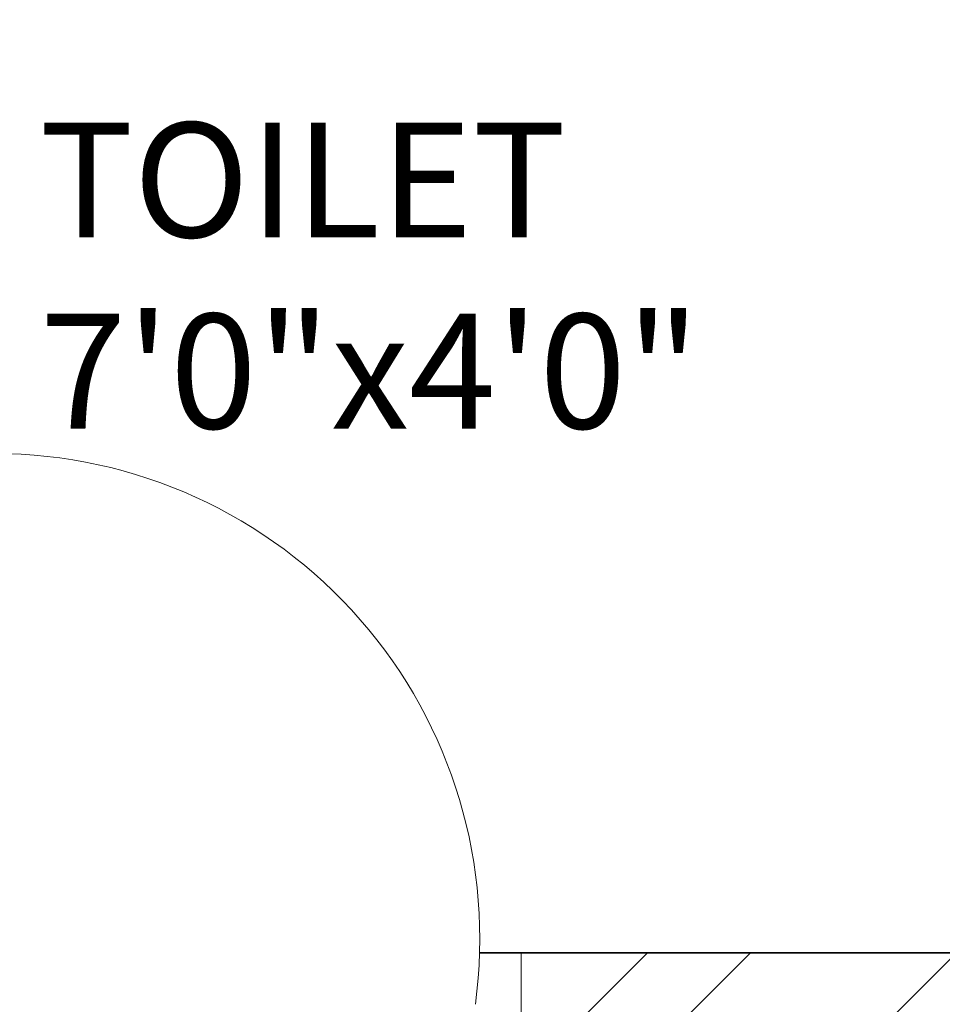
# Model space of a CAD drawing. Units: inches. Extents: x 1962 to 2771, y 1245 to 2660.
# Tile 16 of 114: x 2580 to 2621, y 1649 to 1692. Entities that reach past the tile are written whole.
import ezdxf

# ---------------------------------------------------------------- set-up
doc = ezdxf.new("R2010")
doc.units = ezdxf.units.IN
for name, color, linetype, lineweight in [('A-AREA-IDEN', 7, 'Continuous', 18), ('A-DOOR', 3, 'Continuous', 18), ('A-WALL', 7, 'Continuous', 35), ('A-WALL-PATT', 252, 'Continuous', 13)]:
    doc.layers.add(name, color=color, linetype=linetype, lineweight=lineweight)
doc.styles.get("Standard").update_dxf_attribs({"font": 'arial.ttf'})

msp = doc.modelspace()

# ---------------------------------------------------------------- hatches: boundary and pattern name
at = {"layer": 'A-WALL-PATT'}
h = msp.add_hatch(dxfattribs=at)
h.set_pattern_fill('ANSI32', color=256)
h.paths.add_polyline_path([(2090.8074, 2467.3437), (2141.6481, 2467.3437), (2141.6481, 2469.5937), (2141.6481, 2471.8437), (2086.3074, 2471.8437), (2086.3074, 2422.5333), (2090.8074, 2422.5333)])
h.paths.add_polyline_path([(2282.7664, 2471.8437), (2204.8982, 2471.8437), (2204.8982, 2467.3437), (2234.8074, 2467.3437), (2234.8074, 2311.3437), (2228.7492, 2311.3437), (2228.7492, 2306.8437), (2234.8074, 2306.8437), (2331.9227, 2306.8437), (2331.9227, 2309.0937), (2331.9227, 2311.3437), (2239.3074, 2311.3437), (2239.3074, 2467.3437), (2282.7664, 2467.3437), (2282.7664, 2469.5937)])
h.paths.add_polyline_path([(2471.4531, 2519.8437), (2552.011, 2519.8437), (2564.3996, 2519.8437), (2564.3996, 2511.1389), (2568.8996, 2511.1389), (2568.8996, 2524.3437), (2466.9531, 2524.3437), (2466.9531, 2471.8437), (2450.0749, 2471.8437), (2446.4672, 2471.8437), (2446.4672, 2467.3437), (2450.0749, 2467.3437), (2475.9988, 2467.3437), (2475.9988, 2469.5937), (2475.9988, 2471.8437), (2471.4531, 2471.8437)])
h.paths.add_polyline_path([(2575.2231, 2469.5937), (2575.2231, 2471.8437), (2568.8996, 2471.8437), (2568.8996, 2487.1389), (2564.3996, 2487.1389), (2564.3996, 2471.8437), (2556.511, 2471.8437), (2499.2904, 2471.8437), (2499.2904, 2467.3437), (2507.8074, 2467.3437), (2507.8074, 2311.3437), (2414.863, 2311.3437), (2414.863, 2306.8437), (2512.3074, 2306.8437), (2517.0114, 2306.8437), (2517.0114, 2309.0937), (2517.0114, 2311.3437), (2512.3074, 2311.3437), (2512.3074, 2467.3437), (2575.2231, 2467.3437)])
h.paths.add_polyline_path([(2660.8074, 2471.8437), (2600.9602, 2471.8437), (2600.9602, 2467.3437), (2656.3074, 2467.3437), (2656.3074, 2432.5704), (2660.8074, 2432.5704)])
h.paths.add_polyline_path([(2660.8074, 2372.5704), (2656.3074, 2372.5704), (2656.3074, 2311.3437), (2600.276, 2311.3437), (2600.276, 2309.0937), (2600.276, 2306.8437), (2656.3074, 2306.8437), (2656.3074, 2296.2593), (2660.8074, 2296.2593)])
h.paths.add_polyline_path([(2572.3074, 2306.8437), (2577.1385, 2306.8437), (2577.1385, 2311.3437), (2551.082, 2311.3437), (2551.082, 2306.8437), (2567.8074, 2306.8437), (2567.8074, 2258.8437), (2540.0574, 2258.8437), (2540.0574, 2256.5937), (2540.0574, 2254.3437), (2567.8074, 2254.3437), (2656.3074, 2254.3437), (2656.3074, 2236.9085), (2660.8074, 2236.9085), (2660.8074, 2272.2593), (2656.3074, 2272.2593), (2656.3074, 2258.8437), (2572.3074, 2258.8437)])
h.paths.add_polyline_path([(2512.3074, 2254.3437), (2518.8716, 2254.3437), (2518.8716, 2256.5937), (2518.8716, 2258.8437), (2507.8074, 2258.8437), (2507.8074, 2177.8437), (2567.8074, 2177.8437), (2567.8074, 2172.9628), (2572.3074, 2172.9628), (2572.3074, 2177.8437), (2656.3074, 2177.8437), (2656.3074, 2166.4846), (2660.8074, 2166.4846), (2660.8074, 2200.9085), (2656.3074, 2200.9085), (2656.3074, 2182.3437), (2512.3074, 2182.3437)])
h.paths.add_polyline_path([(2656.3074, 2129.8437), (2572.3074, 2129.8437), (2572.3074, 2150.3044), (2570.0574, 2150.3044), (2567.8074, 2150.3044), (2567.8074, 2129.8437), (2507.8074, 2129.8437), (2507.8074, 2116.3027), (2510.0574, 2116.3027), (2512.3074, 2116.3027), (2512.3074, 2125.3437), (2567.8074, 2125.3437), (2572.3074, 2125.3437), (2656.3074, 2125.3437)])
h.paths.add_polyline_path([(2090.8074, 2362.5333), (2086.3074, 2362.5333), (2086.3074, 2298.6242), (2090.8074, 2298.6242), (2090.8074, 2306.8437), (2174.8074, 2306.8437), (2174.8074, 2286.4178), (2179.3074, 2286.4178), (2179.3074, 2306.8437), (2192.8641, 2306.8437), (2192.8641, 2309.0937), (2192.8641, 2311.3437), (2090.8074, 2311.3437)])
h.paths.add_polyline_path([(2209.156, 2258.8437), (2179.3074, 2258.8437), (2179.3074, 2263.2236), (2177.0574, 2263.2236), (2174.8074, 2263.2236), (2174.8074, 2258.8437), (2090.8074, 2258.8437), (2090.8074, 2274.6242), (2086.3074, 2274.6242), (2086.3074, 2238.2967), (2088.5574, 2238.2967), (2090.8074, 2238.2967), (2090.8074, 2254.3437), (2209.156, 2254.3437)])
h.paths.add_polyline_path([(2090.8074, 2177.8437), (2234.8074, 2177.8437), (2234.8074, 2173.1428), (2239.3074, 2173.1428), (2239.3074, 2258.8437), (2230.8442, 2258.8437), (2230.8442, 2256.5937), (2230.8442, 2254.3437), (2234.8074, 2254.3437), (2234.8074, 2182.3437), (2090.8074, 2182.3437), (2090.8074, 2202.2967), (2086.3074, 2202.2967), (2086.3074, 2140.0389), (2090.8074, 2140.0389)])
h.paths.add_polyline_path([(2090.8074, 2080.0389), (2086.3074, 2080.0389), (2086.3074, 2033.8437), (2090.8074, 2033.8437)], flags=17)
h.paths.add_polyline_path([(2244.9405, 2033.8437), (2239.3074, 2033.8437), (2239.3074, 2142.0665), (2237.2592, 2142.0665), (2234.8074, 2142.0665), (2234.8074, 2033.8437), (2090.8074, 2033.8437), (2076.5204, 2033.8437), (2072.0204, 2033.8437), (2072.0204, 2000.4493), (2076.5204, 2000.4493), (2076.5204, 2029.3437), (2090.8074, 2029.3437), (2244.9405, 2029.3437), (2244.9405, 2031.5937)])
h.paths.add_polyline_path([(2234.8074, 1933.3437), (2076.5204, 1933.3437), (2076.5204, 1952.4493), (2074.2704, 1952.4493), (2072.0204, 1952.4493), (2072.0204, 1933.3437), (2072.0204, 1928.8437), (2234.8074, 1928.8437)])
h.paths.add_polyline_path([(2090.8074, 1928.8437), (2086.3074, 1928.8437), (2086.3074, 1906.5013), (2090.8074, 1906.5013)])
h.paths.add_polyline_path([(2090.8074, 1846.5013), (2086.3074, 1846.5013), (2086.3074, 1769.9917), (2088.5574, 1769.9917), (2090.8074, 1769.9917), (2090.8074, 1780.3437), (2234.8074, 1780.3437), (2234.8074, 1708.3437), (2230.3764, 1708.3437), (2230.3764, 1703.8437), (2239.3074, 1703.8437), (2239.3074, 1792.6669), (2237.0574, 1792.6669), (2234.8074, 1792.6669), (2234.8074, 1784.8437), (2090.8074, 1784.8437)])
h.paths.add_polyline_path([(2239.3074, 1928.8437), (2244.9405, 1928.8437), (2244.9405, 1931.0937), (2244.9405, 1933.3437), (2234.8074, 1933.3437), (2234.8074, 1928.8437), (2234.8074, 1825.5949), (2239.3074, 1825.5949)])
h.paths.add_polyline_path([(2148.0425, 1649.0937), (2148.0425, 1651.3437), (2090.8074, 1651.3437), (2090.8074, 1646.8437), (2148.0425, 1646.8437)], flags=0)
h.paths.add_polyline_path([(2207.5601, 1708.3437), (2090.8074, 1708.3437), (2090.8074, 1703.8437), (2174.8074, 1703.8437), (2174.8074, 1651.3437), (2170.4457, 1651.3437), (2170.4457, 1646.8437), (2195.9924, 1646.8437), (2195.9924, 1649.0937), (2195.9924, 1651.3437), (2179.3074, 1651.3437), (2179.3074, 1703.8437), (2207.5601, 1703.8437), (2207.5601, 1706.0937)])
h.paths.add_polyline_path([(2090.8074, 1733.9917), (2086.3074, 1733.9917), (2086.3074, 1696.1032), (2088.5574, 1696.1032), (2090.8074, 1696.1032)])
h.paths.add_polyline_path([(2090.8074, 1672.1032), (2086.3074, 1672.1032), (2086.3074, 1600.3335), (2090.8074, 1600.3335)])
h.paths.add_polyline_path([(2090.8074, 1540.3335), (2086.3074, 1540.3335), (2086.3074, 1486.3437), (2139.6766, 1486.3437), (2139.6766, 1490.8437), (2090.8074, 1490.8437)])
h.paths.add_polyline_path([(2302.3876, 1490.8437), (2239.3074, 1490.8437), (2239.3074, 1646.8437), (2335.9994, 1646.8437), (2335.9994, 1651.3437), (2229.884, 1651.3437), (2229.884, 1646.8437), (2234.8074, 1646.8437), (2234.8074, 1490.8437), (2202.7103, 1490.8437), (2202.7103, 1488.5937), (2202.7103, 1486.3437), (2275.0699, 1486.3437), (2275.0699, 1475.772), (2279.5699, 1475.772), (2279.5699, 1486.3437), (2302.3876, 1486.3437)])
h.paths.add_polyline_path([(2279.5699, 1451.772), (2275.0699, 1451.772), (2275.0699, 1438.3437), (2174.8074, 1438.3437), (2174.8074, 1486.3437), (2179.7922, 1486.3437), (2179.7922, 1490.8437), (2163.3585, 1490.8437), (2163.3585, 1488.5937), (2163.3585, 1486.3437), (2170.3074, 1486.3437), (2170.3074, 1433.8437), (2279.5699, 1433.8437)])
h.paths.add_polyline_path([(2427.2363, 1490.8437), (2375.8074, 1490.8437), (2375.8074, 1646.8437), (2381.6401, 1646.8437), (2381.6401, 1651.3437), (2365.887, 1651.3437), (2365.887, 1649.0937), (2365.887, 1646.8437), (2371.3074, 1646.8437), (2371.3074, 1490.8437), (2327.5627, 1490.8437), (2327.5627, 1488.5937), (2327.5627, 1486.3437), (2371.3074, 1486.3437), (2371.3074, 1433.8437), (2375.8074, 1433.8437), (2375.8074, 1486.3437), (2427.2363, 1486.3437)])
h.paths.add_polyline_path([(2512.3074, 1646.8437), (2519.4351, 1646.8437), (2519.4351, 1649.0937), (2519.4351, 1651.3437), (2507.8074, 1651.3437), (2416.0063, 1651.3437), (2416.0063, 1649.0937), (2416.0063, 1646.8437), (2507.8074, 1646.8437), (2507.8074, 1490.8437), (2497.0532, 1490.8437), (2497.0532, 1488.5937), (2497.0532, 1486.3437), (2574.9344, 1486.3437), (2574.9344, 1476.0181), (2579.4344, 1476.0181), (2579.4344, 1486.3437), (2584.4872, 1486.3437), (2584.3074, 1490.8437), (2512.3074, 1490.8437)])
h.paths.add_polyline_path([(2470.5091, 1486.3437), (2473.9767, 1486.3437), (2473.9767, 1490.8437), (2449.6605, 1490.8437), (2449.6605, 1488.5937), (2449.6605, 1486.3437), (2466.0091, 1486.3437), (2466.0091, 1433.8437), (2470.5091, 1433.8437), (2579.4344, 1433.8437), (2579.4344, 1452.0181), (2574.9344, 1452.0181), (2574.9344, 1438.3437), (2554.5091, 1438.3437), (2470.5091, 1438.3437)])
h.paths.add_polyline_path([(2656.3074, 1490.8437), (2611.86, 1490.8437), (2611.86, 1486.3437), (2656.3074, 1486.3437)])
h.paths.add_polyline_path([(2660.8074, 1532.7007), (2658.5574, 1532.7007), (2656.3074, 1532.7007), (2656.3074, 1486.3437), (2660.8074, 1486.3437)])
h.paths.add_polyline_path([(2660.8074, 1664.9663), (2656.3074, 1664.9663), (2656.3074, 1651.3437), (2602.2313, 1651.3437), (2602.2313, 1646.8437), (2656.3074, 1646.8437), (2656.3074, 1592.7007), (2660.8074, 1592.7007)])
h.paths.add_polyline_path([(2660.8074, 1724.5221), (2656.3074, 1724.5221), (2656.3074, 1703.8437), (2542.4725, 1703.8437), (2542.4725, 1699.3437), (2567.8074, 1699.3437), (2567.8074, 1651.3437), (2552.7766, 1651.3437), (2552.7766, 1649.0937), (2552.7766, 1646.8437), (2577.2878, 1646.8437), (2577.2878, 1649.0937), (2577.2878, 1651.3437), (2572.3074, 1651.3437), (2572.3074, 1699.3437), (2656.3074, 1699.3437), (2656.3074, 1688.9663), (2660.8074, 1688.9663)])
h.paths.add_polyline_path([(2660.8074, 1880.6524), (2656.3074, 1880.6524), (2656.3074, 1832.8437), (2512.3074, 1832.8437), (2512.3074, 1837.8959), (2507.8074, 1837.8959), (2507.8074, 1828.3437), (2567.8074, 1828.3437), (2567.8074, 1804.3437), (2572.3074, 1804.3437), (2572.3074, 1828.3437), (2656.3074, 1828.3437), (2656.3074, 1818.6778), (2660.8074, 1818.6778)])
h.paths.add_polyline_path([(2660.8074, 1794.6778), (2656.3074, 1794.6778), (2656.3074, 1780.3437), (2572.3074, 1780.3437), (2572.3074, 1783.0303), (2570.0574, 1783.0303), (2567.8074, 1783.0303), (2567.8074, 1780.3437), (2507.8074, 1780.3437), (2507.8074, 1699.3437), (2517.8858, 1699.3437), (2517.8858, 1701.5937), (2517.8858, 1703.8437), (2512.3074, 1703.8437), (2512.3074, 1775.8437), (2656.3074, 1775.8437), (2656.3074, 1760.5221), (2660.8074, 1760.5221)])
h.paths.add_polyline_path([(2660.8074, 1981.3437), (2660.8074, 2020.2808), (2658.5574, 2020.2808), (2656.3074, 2020.2808), (2656.3074, 1981.3437), (2512.3074, 1981.3437), (2512.3074, 2086.6996), (2507.8074, 2086.6996), (2507.8074, 1981.3437), (2375.8074, 1981.3437), (2375.8074, 1986.8505), (2373.5574, 1986.8505), (2371.3074, 1986.8505), (2371.3074, 1973.2607), (2375.8074, 1973.2607), (2375.8074, 1976.8437), (2507.8074, 1976.8437), (2507.8074, 1865.4281), (2510.0574, 1865.4281), (2512.3074, 1865.4281), (2512.3074, 1976.8437), (2660.8074, 1976.8437)])
h.paths.add_polyline_path([(2375.8074, 1940.297), (2373.5574, 1940.297), (2371.3074, 1940.297), (2371.3074, 1933.3437), (2278.4434, 1933.3437), (2278.4434, 1928.8437), (2371.3074, 1928.8437), (2371.3074, 1651.3437), (2375.8074, 1651.3437)])
h.paths.add_polyline_path([(2660.8074, 1976.8437), (2656.3074, 1976.8437), (2656.3074, 1940.6524), (2660.8074, 1940.6524)], flags=17)
h.paths.add_polyline_path([(2660.8074, 2142.4846), (2656.3074, 2142.4846), (2656.3074, 2080.2808), (2660.8074, 2080.2808)])
h.paths.add_polyline_path([(2381.4189, 2311.3437), (2375.8074, 2311.3437), (2375.8074, 2467.3437), (2424.7242, 2467.3437), (2424.7242, 2469.5937), (2424.7242, 2471.8437), (2375.8074, 2471.8437), (2375.8074, 2524.3437), (2371.3074, 2524.3437), (2371.3074, 2471.8437), (2307.2097, 2471.8437), (2307.2097, 2467.3437), (2371.3074, 2467.3437), (2371.3074, 2311.3437), (2366.8901, 2311.3437), (2366.8901, 2306.8437), (2371.3074, 2306.8437), (2371.3074, 2033.8437), (2279.6589, 2033.8437), (2279.6589, 2029.3437), (2371.3074, 2029.3437), (2371.3074, 2014.2598), (2375.8074, 2014.2598), (2375.8074, 2306.8437), (2381.4189, 2306.8437)])
h.paths.add_polyline_path([(2263.3074, 2524.3437), (2170.3074, 2524.3437), (2170.3074, 2519.8437), (2170.3074, 2471.8437), (2165.0312, 2471.8437), (2165.0312, 2467.3437), (2179.6721, 2467.3437), (2179.6721, 2469.5161), (2179.6721, 2471.8437), (2174.8074, 2471.8437), (2174.8074, 2519.8437), (2258.8074, 2519.8437), (2258.8074, 2511.6436), (2263.3074, 2511.6436)])
h.paths.add_polyline_path([(2245.0232, 1361.4123), (2492.9468, 1361.4123), (2492.9468, 1398.505), (2245.0232, 1398.505)], flags=9)
h.paths.add_polyline_path([(2388.1434, 2086.6936), (2425.0704, 2086.6936), (2425.0704, 2105.3509), (2388.1434, 2105.3509)], flags=9)
h.paths.add_polyline_path([(2404.922, 2242.6744), (2445.7337, 2242.6744), (2445.7337, 2261.3318), (2404.922, 2261.3318)], flags=9)
h.paths.add_polyline_path([(2269.4107, 2156.7935), (2306.3378, 2156.7935), (2306.3378, 2175.4508), (2269.4107, 2175.4508)], flags=9)
h.paths.add_polyline_path([(2269.3277, 2233.4343), (2306.2547, 2233.4343), (2306.2547, 2252.0917), (2269.3277, 2252.0917)], flags=9)
h.paths.add_polyline_path([(2431.6052, 2320.6922), (2470.4456, 2320.6922), (2470.4456, 2339.3495), (2431.6052, 2339.3495)], flags=25)
h.paths.add_polyline_path([(2249.6902, 2315.7608), (2288.5306, 2315.7608), (2288.5306, 2334.4182), (2249.6902, 2334.4182)], flags=25)
h.paths.add_polyline_path([(2096.9301, 2314.3181), (2135.7704, 2314.3181), (2135.7704, 2332.9755), (2096.9301, 2332.9755)], flags=25)
h.paths.add_polyline_path([(2134.3475, 2285.7089), (2161.4655, 2285.7089), (2161.4655, 2304.3662), (2134.3475, 2304.3662)], flags=9)
h.paths.add_polyline_path([(2126.5155, 2209.4076), (2159.9227, 2209.4076), (2159.9227, 2228.065), (2126.5155, 2228.065)], flags=25)
h.paths.add_polyline_path([(2110.5753, 2141.5299), (2149.4157, 2141.5299), (2149.4157, 2160.1872), (2110.5753, 2160.1872)], flags=25)
h.paths.add_polyline_path([(2249.8618, 1968.3317), (2286.3966, 1968.3317), (2286.3966, 1986.989), (2249.8618, 1986.989)], flags=9)
h.paths.add_polyline_path([(2395.9507, 1777.0051), (2436.7624, 1777.0051), (2436.7624, 1795.6625), (2395.9507, 1795.6625)], flags=9)
h.paths.add_polyline_path([(2398.5259, 1888.5651), (2435.0062, 1888.5651), (2435.0062, 1907.2224), (2398.5259, 1907.2224)], flags=25)
h.paths.add_polyline_path([(2259.3506, 1728.3559), (2296.2776, 1728.3559), (2296.2776, 1747.0132), (2259.3506, 1747.0132)], flags=9)
h.paths.add_polyline_path([(2271.3698, 1845.268), (2308.2968, 1845.268), (2308.2968, 1863.9253), (2271.3698, 1863.9253)], flags=9)
h.paths.add_polyline_path([(2120.9355, 1786.3027), (2159.7759, 1786.3027), (2159.7759, 1804.9601), (2120.9355, 1804.9601)], flags=25)
h.paths.add_polyline_path([(2121.3164, 1732.1043), (2154.7236, 1732.1043), (2154.7236, 1750.7616), (2121.3164, 1750.7616)], flags=25)
h.paths.add_polyline_path([(2118.3706, 1678.8997), (2147.5282, 1678.8997), (2147.5282, 1697.557), (2118.3706, 1697.557)], flags=25)
h.paths.add_polyline_path([(2385.9227, 1493.557), (2424.763, 1493.557), (2424.763, 1512.2143), (2385.9227, 1512.2143)], flags=25)
h.paths.add_polyline_path([(2248.7058, 1500.0256), (2287.5462, 1500.0256), (2287.5462, 1518.6829), (2248.7058, 1518.6829)], flags=25)
h.paths.add_polyline_path([(2104.1669, 1617.3771), (2143.0073, 1617.3771), (2143.0073, 1636.0344), (2104.1669, 1636.0344)], flags=9)
h.paths.add_polyline_path([(2096.0714, 1447.8824), (2137.3845, 1447.8824), (2137.3845, 1458.1859), (2096.0714, 1458.1859)], flags=9)
h.paths.add_polyline_path([(2180.6114, 1440.325), (2209.7689, 1440.325), (2209.7689, 1458.9823), (2180.6114, 1458.9823)], flags=25)
h.paths.add_polyline_path([(2316.1698, 1447.9637), (2357.4829, 1447.9637), (2357.4829, 1458.2673), (2316.1698, 1458.2673)], flags=9)
h.paths.add_polyline_path([(2397.6187, 1447.9637), (2438.9318, 1447.9637), (2438.9318, 1458.2673), (2397.6187, 1458.2673)], flags=9)
h.paths.add_polyline_path([(2473.0778, 1439.5953), (2502.2354, 1439.5953), (2502.2354, 1458.2527), (2473.0778, 1458.2527)], flags=25)
h.paths.add_polyline_path([(2589.7027, 1447.8819), (2631.0158, 1447.8819), (2631.0158, 1458.1855), (2589.7027, 1458.1855)], flags=9)
h.paths.add_polyline_path([(2522.4009, 1497.5285), (2561.2413, 1497.5285), (2561.2413, 1516.1859), (2522.4009, 1516.1859)], flags=25)
h.paths.add_polyline_path([(2579.6565, 1671.3482), (2608.8141, 1671.3482), (2608.8141, 1690.0056), (2579.6565, 1690.0056)], flags=25)
h.paths.add_polyline_path([(2544.7038, 1725.5064), (2578.1111, 1725.5064), (2578.1111, 1744.1637), (2544.7038, 1744.1637)], flags=25)
h.paths.add_polyline_path([(2578.1191, 1807.472), (2607.2766, 1807.472), (2607.2766, 1826.1293), (2578.1191, 1826.1293)], flags=25)
h.paths.add_polyline_path([(2595.0614, 1835.1839), (2633.9018, 1835.1839), (2633.9018, 1853.8413), (2595.0614, 1853.8413)], flags=25)
h.paths.add_polyline_path([(2567.0097, 2097.7035), (2605.8501, 2097.7035), (2605.8501, 2116.3609), (2567.0097, 2116.3609)], flags=9)
h.paths.add_polyline_path([(2586.644, 2134.6454), (2615.8015, 2134.6454), (2615.8015, 2153.3027), (2586.644, 2153.3027)], flags=9)
h.paths.add_polyline_path([(2544.6185, 2212.6783), (2578.0258, 2212.6783), (2578.0258, 2231.3356), (2544.6185, 2231.3356)], flags=25)
h.paths.add_polyline_path([(2577.0273, 2256.9023), (2606.1849, 2256.9023), (2606.1849, 2275.5597), (2577.0273, 2275.5597)], flags=24)
h.paths.add_polyline_path([(2605.2683, 2315.2821), (2644.1087, 2315.2821), (2644.1087, 2333.9395), (2605.2683, 2333.9395)], flags=25)
h.paths.add_polyline_path([(2583.1244, 2496.1815), (2624.4375, 2496.1815), (2624.4375, 2506.4851), (2583.1244, 2506.4851)], flags=9)
h.paths.add_polyline_path([(2474.761, 2497.0823), (2503.9185, 2497.0823), (2503.9185, 2515.7397), (2474.761, 2515.7397)], flags=25)
h.paths.add_polyline_path([(2387.5787, 2494.2563), (2428.902, 2494.2563), (2428.902, 2504.5598), (2387.5787, 2504.5598)], flags=9)
h.paths.add_polyline_path([(2300.1657, 2500.1564), (2341.4788, 2500.1564), (2341.4788, 2510.46), (2300.1657, 2510.46)], flags=25)
h.paths.add_polyline_path([(2176.8589, 2497.5843), (2206.0165, 2497.5843), (2206.0165, 2516.2416), (2176.8589, 2516.2416)], flags=25)
h.paths.add_polyline_path([(2097.4668, 2494.9762), (2138.7799, 2494.9762), (2138.7799, 2505.2798), (2097.4668, 2505.2798)], flags=9)

# ---------------------------------------------------------------- linework, layer by layer
at = {"layer": 'A-DOOR'}
msp.add_line((2602.2313, 1651.3437), (2602.2313, 1646.8437), dxfattribs=at)
msp.add_arc((2579.2878, 1651.9556), 21.1381, 352.21873, 90, dxfattribs=at)
at = {"layer": 'A-WALL'}
msp.add_line((2656.3074, 1651.3437), (2600.4171, 1651.3437), dxfattribs=at)

# ---------------------------------------------------------------- texts
at = {"layer": 'A-AREA-IDEN', "insert": (2581.2374, 1687.5209), "char_height": 5, "attachment_point": 1}
msp.add_mtext_dynamic_manual_height_columns('TOILET\\P7\'0"x4\'0"', width=111.820054, gutter_width=12.5, heights=[0], dxfattribs=at)

doc.saveas('drawing.dxf')
